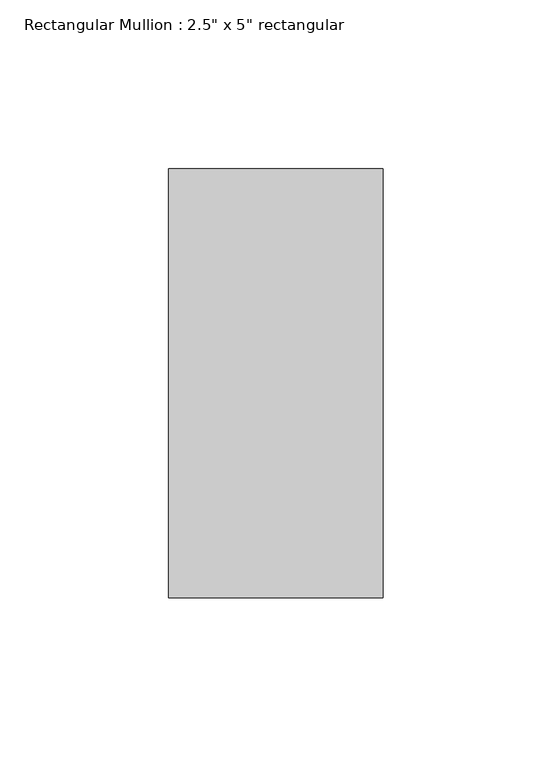
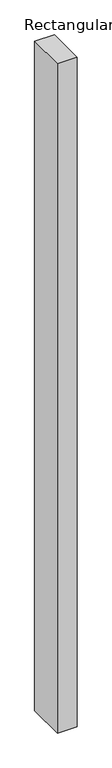
"""IFC4 building model written with IfcOpenShell, lengths in millimetres: member geometry."""

from ifc_helpers import new_model, si_unit, frame, origin, place, context, project, spatial, polyline, outline, extrude, source, transform, mapped, element, save


def member_860c46db(model_context):
    return source(origin(), model_context, "Body", "SweptSolid", [
        extrude(outline(polyline([(0.0, 63.5), (0.0, -63.5), (-63.5, -63.5), (-63.5, 63.5), (0.0, 63.5)])), frame((0.0, 0.0, -2286.0), z_axis=(0.0, 0.0, 1.0), x_axis=(1.0, 0.0, 0.0)), (0.0, 0.0, 1.0), 2286.0),
    ])


if __name__ == "__main__":
    model = new_model("IFC4")
    model_context = context("Model", 3, world=origin())
    ifc_project = project(units=[si_unit("LENGTHUNIT", "METRE", prefix="MILLI")], contexts=[model_context])
    site = spatial("IfcSite", under=ifc_project)
    building = spatial("IfcBuilding", under=site)
    placement = place(None, origin())
    member_shape = member_860c46db(model_context)
    element("IfcMember", 1, ObjectType="Rectangular Mullion : 2.5\" x 5\" rectangular", at=placement, inside=building, context=model_context, shape_type="MappedRepresentation", body=[
        mapped(member_shape, transform((0.0, 0.0, 0.0), x_axis=(1.0, 0.0, 0.0), y_axis=(0.0, 1.0, 0.0), z_axis=(0.0, 0.0, 1.0))),
    ])
    save(model, "model.ifc")

# Revit data of these elements
# Type "Rectangular Mullion : 2.5\" x 5\" rectangular"
#   built-in parameter 1007304 = 0.416667 (stored number, unit not read)
#   built-in parameter 1007301 = 0.104167 (stored number, unit not read)
#   built-in parameter 1007300 = 0.104167 (stored number, unit not read)
# Element 1 (IfcMember, "Rectangular Mullion : 2.5\" x 5\" rectangular")
#   Materials on its faces: "Aluminum"
# Materials
#   "Aluminum": class "Metal", colour RGB 247 247 247, transparency 0, Description = "Aluminum 6061", Cost = 0
